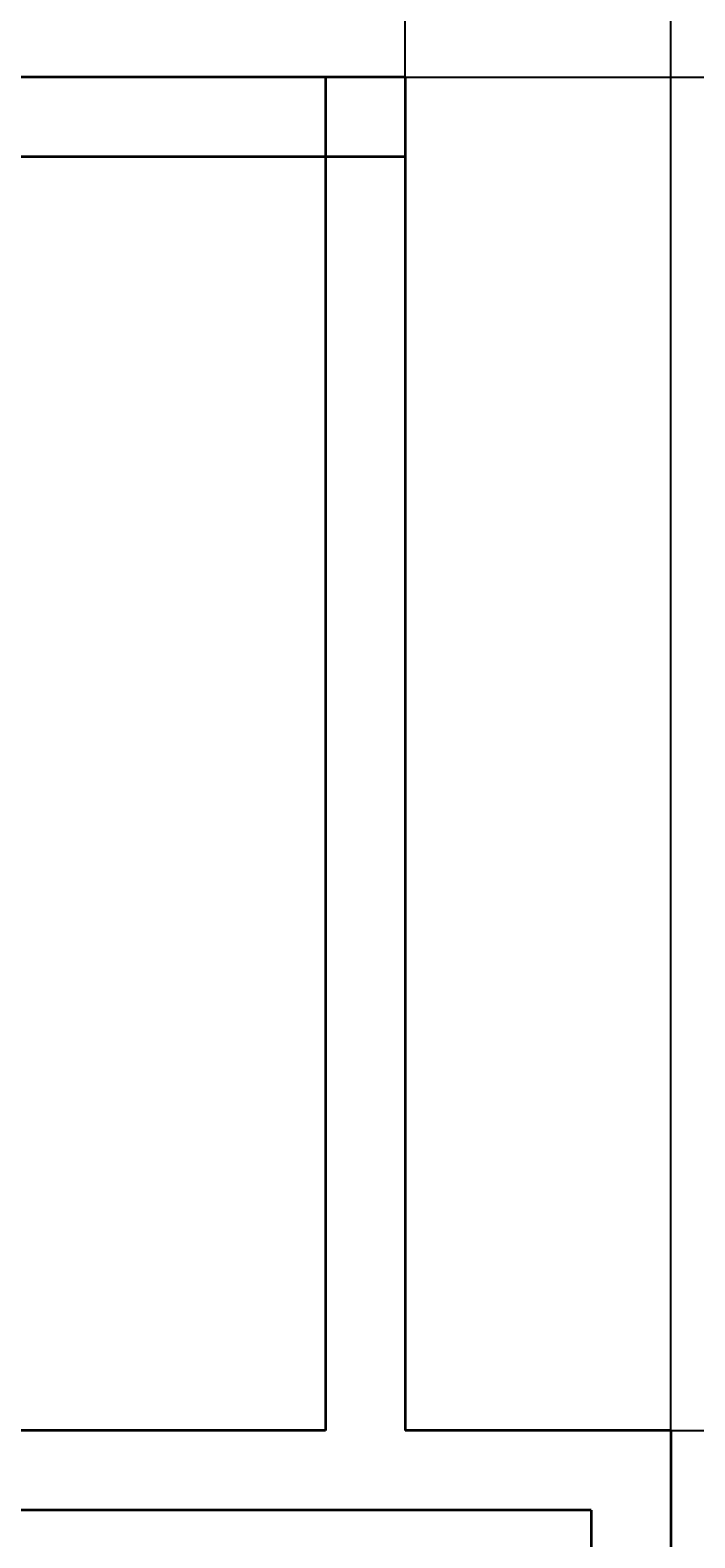
# Model space of a CAD drawing. Units: inches. Extents: x 867 to 1667, y -234 to 788.
# Tile 40 of 42: x 1497 to 1572, y 401 to 572. Entities that reach past the tile are written whole.
import ezdxf

# ---------------------------------------------------------------- set-up
doc = ezdxf.new("R2010")
doc.units = ezdxf.units.IN
doc.header["$MEASUREMENT"] = 0
doc.layers.add('A-ANNO-DIMS', color=2, linetype='Continuous', lineweight=18)
doc.layers.add('A-Wall', color=7, linetype='Continuous', lineweight=35)
doc.styles.get("Standard").update_dxf_attribs({"font": 'arial.ttf'})
doc.dimstyles.get("Standard").update_dxf_attribs({"dimtxt": 0.6875, "dimasz": 0.18, "dimexe": 0.18, "dimexo": 0.0625, "dimgap": 0.09, "dimtad": 0, "dimdec": 4, "dimzin": 0, "dimdsep": 46, "dimlunit": 4, "dimtxsty": 'Standard', "dimcen": 0.09, "dimadec": 0, "dimazin": 0, "dimtfac": 1, "dimtdec": 4, "dimtofl": 0, "dimtmove": 0, "dimatfit": 3, "dimfxl": 1, "dimtolj": 1, "dimtzin": 0, "dimarcsym": 0})

# ---------------------------------------------------------------- blocks, each defined once
blk = doc.blocks.new('*D31')
at = {"layer": 'A-ANNO-DIMS', "color": 0, "lineweight": -2, "transparency": 16777216}
for p, q in [((1070.89, 566.68), (1070.89, 787.75)), ((1071.07, 787.57), (1304.02, 787.57)), ((1538.71, 787.57), (1305.75, 787.57)), ((1538.89, 566.68), (1538.89, 787.75))]:
    blk.add_line(p, q, dxfattribs=at)
at = {"layer": 'A-ANNO-DIMS', "color": 0, "transparency": 16777216}
for points in [[(1071.07, 787.6), (1071.07, 787.54), (1070.89, 787.57)], [(1538.71, 787.6), (1538.71, 787.54), (1538.89, 787.57)]]:
    blk.add_solid(points, dxfattribs=at)
at = {"layer": 'Defpoints', "color": 0, "transparency": 16777216}
for p in [(1538.89, 787.57), (1070.89, 566.62), (1538.89, 566.62)]:
    blk.add_point(p, dxfattribs=at)
at = {"layer": 'A-ANNO-DIMS', "color": 0, "transparency": 16777216, "insert": (1304.89, 787.57), "char_height": 0.688, "attachment_point": 5}
blk.add_mtext('\\A1;468', dxfattribs=at)
blk = doc.blocks.new('*D34')
at = {"layer": 'A-ANNO-DIMS', "color": 0, "lineweight": -2, "transparency": 16777216}
for p, q in [((1538.95, 566.62), (1667.02, 566.62)), ((1666.84, 566.44), (1666.84, 490.93)), ((1666.84, 413.8), (1666.84, 489.3)), ((1538.95, 413.62), (1667.02, 413.62))]:
    blk.add_line(p, q, dxfattribs=at)
at = {"layer": 'A-ANNO-DIMS', "color": 0, "transparency": 16777216}
for points in [[(1666.81, 566.44), (1666.87, 566.44), (1666.84, 566.62)], [(1666.81, 413.8), (1666.87, 413.8), (1666.84, 413.62)]]:
    blk.add_solid(points, dxfattribs=at)
at = {"layer": 'Defpoints', "color": 0, "transparency": 16777216}
for p in [(1538.89, 566.62), (1666.84, 566.62), (1538.89, 413.62)]:
    blk.add_point(p, dxfattribs=at)
at = {"layer": 'A-ANNO-DIMS', "color": 0, "transparency": 16777216, "insert": (1666.84, 490.12), "char_height": 0.688, "attachment_point": 5, "rotation": 90}
blk.add_mtext('\\A1;153', dxfattribs=at)
blk = doc.blocks.new('*D36')
at = {"layer": 'A-ANNO-DIMS', "color": 0, "lineweight": -2, "transparency": 16777216}
for p, q in [((1538.89, 413.68), (1538.89, 787.75)), ((1539.07, 787.57), (1553.31, 787.57)), ((1568.71, 787.57), (1554.47, 787.57)), ((1568.89, 413.68), (1568.89, 787.75))]:
    blk.add_line(p, q, dxfattribs=at)
at = {"layer": 'A-ANNO-DIMS', "color": 0, "transparency": 16777216}
for points in [[(1539.07, 787.6), (1539.07, 787.54), (1538.89, 787.57)], [(1568.71, 787.6), (1568.71, 787.54), (1568.89, 787.57)]]:
    blk.add_solid(points, dxfattribs=at)
at = {"layer": 'Defpoints', "color": 0, "transparency": 16777216}
for p in [(1568.89, 787.57), (1538.89, 413.62), (1568.89, 413.62)]:
    blk.add_point(p, dxfattribs=at)
at = {"layer": 'A-ANNO-DIMS', "color": 0, "transparency": 16777216, "insert": (1553.89, 787.57), "char_height": 0.688, "attachment_point": 5}
blk.add_mtext('\\A1;30', dxfattribs=at)

msp = doc.modelspace()

# ---------------------------------------------------------------- linework, layer by layer
at = {"layer": 'A-Wall'}
for p, q in [((1538.8866, 566.617), (1070.8866, 566.617)), ((1529.8866, 566.617), (1529.8866, 413.617)), ((1538.8866, 566.617), (1538.8866, 413.617)), ((1538.8866, 557.617), (1070.8866, 557.617)), ((1529.8866, 413.617), (1040.8866, 413.617)), ((1568.8866, 413.617), (1538.8866, 413.617)), ((1568.8866, 413.617), (1568.8866, 257.617)), ((1559.8866, 404.617), (1040.8866, 404.617)), ((1559.8866, 404.617), (1559.8866, 257.617))]:
    msp.add_line(p, q, dxfattribs=at)

# ---------------------------------------------------------------- dimensions: what is measured, and where the dimension line sits
at = {"layer": 'A-ANNO-DIMS'}
for base, p1, p2, picture, middle in [((1538.8866, 787.567), (1070.8866, 566.617), (1538.8866, 566.617), '*D31', (1304.8866, 787.567)), ((1568.8866, 787.567), (1538.8866, 413.617), (1568.8866, 413.617), '*D36', (1553.8866, 787.567))]:
    dim = msp.add_linear_dim(base=base, p1=p1, p2=p2, dimstyle='Standard', override={"dimdec": 0, "dimlfac": 1, "dimrnd": 0, "dimzin": 0, "dimdsep": 46, "dimlunit": 2}, dxfattribs=at)
    dim.commit()
    dim.dimension.update_dxf_attribs({"geometry": picture, "text_midpoint": middle})
dim = msp.add_linear_dim(base=(1666.8366, 566.617), p1=(1538.8866, 413.617), p2=(1538.8866, 566.617), angle=90, dimstyle='Standard', override={"dimdec": 0, "dimlfac": 1, "dimrnd": 0, "dimzin": 0, "dimdsep": 46, "dimlunit": 2}, dxfattribs=at)
dim.commit()
dim.dimension.update_dxf_attribs({"geometry": '*D34', "text_midpoint": (1666.8366, 490.117)})

doc.saveas('drawing.dxf')
